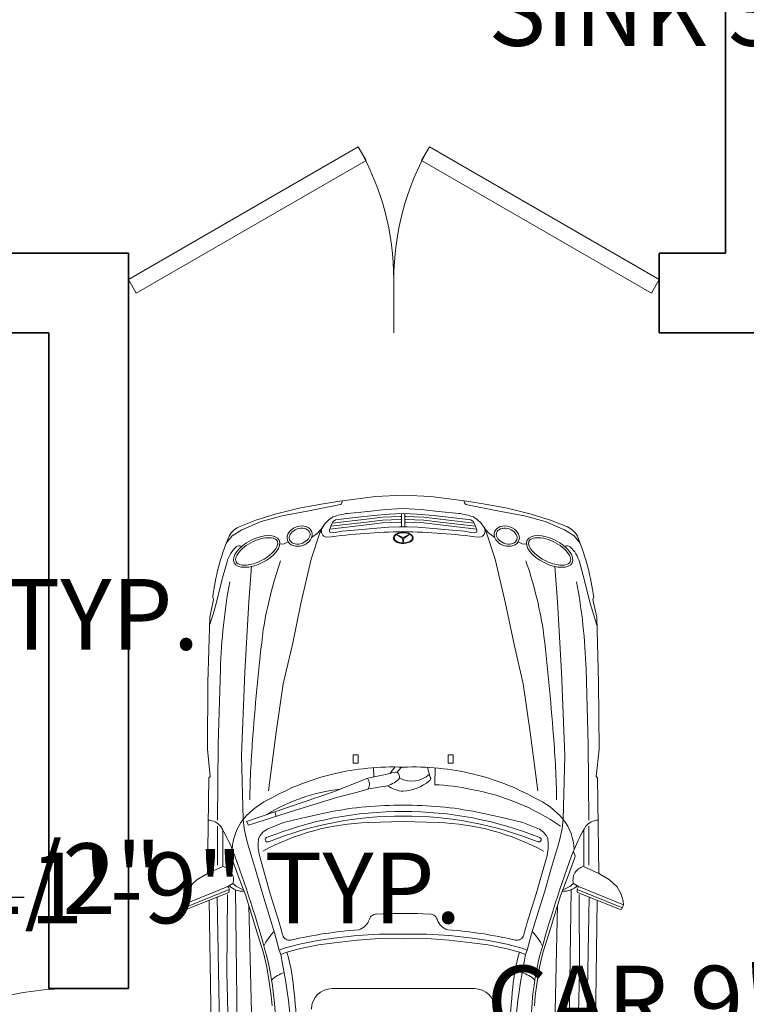
# Model space of a CAD drawing. Units: inches. Extents: x 2558 to 3026, y 433 to 1053.
# Tile 4 of 8: x 2795 to 2877, y 574 to 685. Entities that reach past the tile are written whole.
import ezdxf

# ---------------------------------------------------------------- set-up
doc = ezdxf.new("R2010")
doc.units = ezdxf.units.IN
for name, color, linetype, lineweight in [('0_Equip', 250, 'Continuous', 13), ('A-ANNO-DIMS', 2, 'Continuous', 18), ('A-DOOR', 4, 'Continuous', 18), ('A-WALL', 7, 'Continuous', 35)]:
    doc.layers.add(name, color=color, linetype=linetype, lineweight=lineweight)
doc.styles.get("Standard").update_dxf_attribs({"font": 'arial.ttf'})
doc.dimstyles.new('ISO-25', dxfattribs={"dimtxt": 8, "dimasz": 4, "dimexe": 1, "dimexo": 1, "dimgap": 1, "dimtad": 0, "dimtih": 1, "dimtoh": 1, "dimlunit": 3, "dimtxsty": 'Standard', "dimblk": 'OBLIQUE', "dimcen": 2.5, "dimclrt": 1, "dimadec": 0, "dimazin": 0, "dimtfac": 1, "dimtmove": 0, "dimatfit": 3, "dimfxl": 1, "dimfxlon": 1, "dimarcsym": 0})

# ---------------------------------------------------------------- blocks, each defined once
blk = doc.blocks.new('*U10')
for p, q in [((0, 0), (0, -6)), ((30, 0), (30, -6))]:
    blk.add_line(p, q)
blk.add_lwpolyline([(0, 0), (25.98, 15), (26.86, 13.48), (0.87, -1.52)], close=True)
blk.add_arc((0, 0), 30, 0, 30)
blk = doc.blocks.new('*U4')
for p, q in [((-30, 0), (-30, -6)), ((0, 0), (0, -6))]:
    blk.add_line(p, q)
blk.add_lwpolyline([(0, 0), (-25.98, 15), (-26.86, 13.48), (-0.88, -1.52)], close=True)
blk.add_arc((0, 0), 30, 150, 180)
blk = doc.blocks.new('*U8')
for p, q in [((0, 0), (0, -6)), ((36, 0), (36, -6))]:
    blk.add_line(p, q)
blk.add_lwpolyline([(0, 0), (31.18, 18), (32.05, 16.48), (0.87, -1.52)], close=True)
blk.add_arc((0, 0), 36, 0, 30)
blk = doc.blocks.new('A$C4C7B54D1')
at = {"layer": '0_Equip', "ltscale": 0.1}
for p, q in [((-0.7257, 2.678), (-0.8531, 2.6707)), ((-0.7257, 2.678), (-0.5983, 2.6707)), ((-1.112, 2.6343), (-1.2037, 2.6168)), ((-1.0138, 2.6343), (-1.1673, 2.6045)), ((-1.0176, 2.6505), (-1.112, 2.6343)), ((-0.8531, 2.6707), (-1.0176, 2.6505)), ((-0.5983, 2.6707), (-0.4338, 2.6505)), ((-0.4376, 2.6343), (-0.284, 2.6045)), ((-0.4338, 2.6505), (-0.3394, 2.6343)), ((-0.3394, 2.6343), (-0.2477, 2.6168)), ((-1.3142, 2.5898), (-1.4032, 2.5628)), ((-1.2824, 2.5829), (-1.3789, 2.557)), ((-1.2037, 2.6168), (-1.3142, 2.5898)), ((-1.1673, 2.6045), (-1.2824, 2.5829)), ((-0.8877, 2.6027), (-0.9812, 2.5937)), ((-0.8072, 2.6112), (-0.8877, 2.6027)), ((-0.7257, 2.6157), (-0.8072, 2.6112)), ((-0.7257, 2.6157), (-0.6441, 2.6112)), ((-0.6441, 2.6112), (-0.5636, 2.6027)), ((-0.5636, 2.6027), (-0.4701, 2.5937)), ((-0.284, 2.6045), (-0.1689, 2.5829)), ((-0.2477, 2.6168), (-0.1371, 2.5898)), ((-0.1689, 2.5829), (-0.0725, 2.557)), ((-0.1371, 2.5898), (-0.0481, 2.5628)), ((-1.4032, 2.5628), (-1.4801, 2.5318)), ((-1.3789, 2.557), (-1.4667, 2.5181)), ((-0.0725, 2.557), (0.0153, 2.5181)), ((-0.0481, 2.5628), (0.0288, 2.5318)), ((-1.5113, 2.4907), (-1.5393, 2.4562)), ((-1.4667, 2.5181), (-1.5113, 2.4907)), ((-1.1083, 2.5037), (-1.1486, 2.3827)), ((-0.343, 2.5037), (-0.3027, 2.3827)), ((0.0153, 2.5181), (0.06, 2.4907)), ((0.06, 2.4907), (0.0879, 2.4562)), ((-1.5353, 2.3701), (-1.5529, 2.308)), ((-1.1486, 2.3827), (-1.1961, 2.1797)), ((-0.3027, 2.3827), (-0.2552, 2.1797)), ((0.084, 2.3701), (0.1016, 2.308)), ((-1.435, 2.1869), (-1.4221, 2.3511)), ((-0.0163, 2.1869), (-0.0293, 2.3511)), ((-1.5529, 2.308), (-1.5677, 2.2486)), ((0.1016, 2.308), (0.1164, 2.2486)), ((-1.5677, 2.2486), (-1.5849, 2.1795)), ((0.1164, 2.2486), (0.1336, 2.1795)), ((-1.597, 2.1976), (-1.615, 2.1169)), ((-1.6012, 2.2082), (-1.597, 2.1976)), ((-1.5849, 2.1795), (-1.5997, 2.1304)), ((-1.4537, 1.863), (-1.435, 2.1869)), ((-1.1961, 2.1797), (-1.2349, 1.9911)), ((-0.2552, 2.1797), (-0.2164, 1.9911)), ((0.0024, 1.863), (-0.0163, 2.1869)), ((0.1336, 2.1795), (0.1484, 2.1304)), ((0.1499, 2.2082), (0.1457, 2.1976)), ((0.1457, 2.1976), (0.1637, 2.1169)), ((-1.5997, 2.1304), (-1.6161, 2.0798)), ((0.1484, 2.1304), (0.1647, 2.0798)), ((-1.615, 2.1169), (-1.6235, 1.8165)), ((0.1637, 2.1169), (0.1722, 1.8165)), ((-1.2349, 1.9911), (-1.2767, 1.8097)), ((-0.2164, 1.9911), (-0.1746, 1.8097)), ((-1.566, 1.8774), (-1.5761, 1.5304)), ((-1.4681, 1.48), (-1.4537, 1.863)), ((0.0168, 1.48), (0.0024, 1.863)), ((0.1147, 1.8774), (0.1247, 1.5304)), ((-1.6235, 1.8165), (-1.6256, 1.5098)), ((0.1722, 1.8165), (0.1743, 1.5098)), ((-1.2767, 1.8097), (-1.3098, 1.588)), ((-0.1746, 1.8097), (-0.1415, 1.588)), ((-1.3098, 1.588), (-1.3443, 1.3187)), ((-0.1415, 1.588), (-0.107, 1.3187)), ((-1.6256, 1.5098), (-1.6129, 1.3846)), ((-1.5761, 1.5304), (-1.5789, 1.1834)), ((0.1247, 1.5304), (0.1276, 1.1834)), ((0.1743, 1.5098), (0.1616, 1.3846)), ((-1.461, 1.1868), (-1.4681, 1.48)), ((-0.955, 1.4459), (-0.955, 1.4827)), ((-0.955, 1.4827), (-0.9321, 1.4827)), ((-0.9321, 1.4827), (-0.9321, 1.4459)), ((-0.5192, 1.4827), (-0.5192, 1.4459)), ((-0.4964, 1.4827), (-0.5192, 1.4827)), ((-0.4964, 1.4459), (-0.4964, 1.4827)), ((0.0097, 1.1868), (0.0168, 1.48)), ((-0.9321, 1.4459), (-0.955, 1.4459)), ((-0.8614, 1.4242), (-0.8603, 1.382)), ((-0.6135, 1.4258), (-0.6012, 1.3814)), ((-0.5809, 1.3459), (-0.5793, 1.4233)), ((-0.5192, 1.4459), (-0.4964, 1.4459)), ((-1.6193, 1.3782), (-1.6252, 0.9375)), ((-1.6129, 1.3846), (-1.6193, 1.3782)), ((-0.8878, 1.3764), (-1.0456, 1.313)), ((-0.7861, 1.3973), (-0.8878, 1.3764)), ((0.1616, 1.3846), (0.1679, 1.3782)), ((0.1679, 1.3782), (0.1739, 0.9375)), ((-1.0456, 1.313), (-1.4462, 1.1776)), ((-0.9361, 1.3119), (-0.8835, 1.3269)), ((-0.8835, 1.3269), (-0.7975, 1.3408)), ((-1.2207, 1.2292), (-1.0263, 1.2883)), ((-1.0263, 1.2883), (-0.9361, 1.3119)), ((-1.4366, 1.1604), (-1.2207, 1.2292)), ((-1.4565, 1.1447), (-1.461, 1.1868)), ((-1.4462, 1.1776), (-1.4366, 1.1604)), ((-1.3162, 1.2215), (-1.3088, 1.2011)), ((-1.1723, 1.1976), (-1.2762, 1.1716)), ((-1.0667, 1.22), (-1.1723, 1.1976)), ((-0.7257, 1.1776), (-0.8858, 1.1725)), ((-0.7257, 1.1776), (-0.5655, 1.1725)), ((-0.3847, 1.22), (-0.279, 1.1976)), ((-0.279, 1.1976), (-0.1751, 1.1716)), ((0.0052, 1.1447), (0.0097, 1.1868)), ((-1.5793, 1.1562), (-1.5793, 0.9761)), ((-1.5552, 1.139), (-1.5552, 0.9693)), ((-1.4503, 1.1151), (-1.4565, 1.1447)), ((-1.3515, 1.142), (-1.3703, 1.1286)), ((-1.2762, 1.1716), (-1.3515, 1.142)), ((-0.1751, 1.1716), (-0.0999, 1.142)), ((-0.0999, 1.142), (-0.0811, 1.1286)), ((-0.0011, 1.1151), (0.0052, 1.1447)), ((0.1038, 1.139), (0.1038, 0.9693)), ((0.128, 1.1562), (0.128, 0.9761)), ((-1.444, 1.0892), (-1.4503, 1.1151)), ((-1.4368, 1.0623), (-1.444, 1.0892)), ((-1.39, 1.0981), (-1.3927, 1.0739)), ((-1.3828, 1.1133), (-1.39, 1.0981)), ((-1.3703, 1.1286), (-1.3828, 1.1133)), ((-0.0811, 1.1286), (-0.0685, 1.1133)), ((-0.0685, 1.1133), (-0.0614, 1.0981)), ((-0.0614, 1.0981), (-0.0587, 1.0739)), ((-0.0145, 1.0623), (-0.0073, 1.0892)), ((-0.0073, 1.0892), (-0.0011, 1.1151)), ((-1.4243, 1.0229), (-1.4368, 1.0623)), ((-1.3927, 1.0739), (-1.3918, 1.0533)), ((-1.3918, 1.0533), (-1.3867, 1.0211)), ((-0.0596, 1.0533), (-0.0646, 1.0211)), ((-0.0587, 1.0739), (-0.0596, 1.0533)), ((-0.027, 1.0229), (-0.0145, 1.0623)), ((-1.5149, 1.011), (-1.4844, 0.9277)), ((-1.4064, 0.961), (-1.4243, 1.0229)), ((-1.3867, 1.0211), (-1.3374, 0.8446)), ((-0.0646, 1.0211), (-0.1139, 0.8446)), ((-0.0449, 0.961), (-0.027, 1.0229)), ((0.0635, 1.011), (0.0331, 0.9277)), ((-1.6252, 0.9375), (-1.5546, 0.9696)), ((-1.3759, 0.8562), (-1.4064, 0.961)), ((-0.0754, 0.8562), (-0.0449, 0.961)), ((0.1739, 0.9375), (0.1032, 0.9696)), ((-1.6745, 0.908), (-1.7088, 0.8764)), ((-1.6252, 0.9375), (-1.6745, 0.908)), ((-1.4844, 0.9277), (-1.4486, 0.8345)), ((0.0331, 0.9277), (-0.0028, 0.8345)), ((0.1739, 0.9375), (0.2232, 0.908)), ((0.2232, 0.908), (0.2574, 0.8764)), ((-1.5321, 0.8786), (-1.7381, 0.7945)), ((-1.5253, 0.865), (-1.7329, 0.7802)), ((-1.7088, 0.8764), (-1.728, 0.8432)), ((-1.508, 0.8914), (-1.5321, 0.8786)), ((-1.4835, -0.0735), (-1.497, 0.863)), ((0.0322, -0.0735), (0.0457, 0.863)), ((0.0566, 0.8914), (0.0807, 0.8786)), ((0.074, 0.865), (0.2816, 0.7802)), ((0.0807, 0.8786), (0.2867, 0.7945)), ((0.2574, 0.8764), (0.2767, 0.8432)), ((-1.728, 0.8432), (-1.7366, 0.8127)), ((-1.5273, 0.8512), (-1.7203, 0.7738)), ((-1.6171, 0.8152), (-1.5964, -0.6171)), ((-1.5805, 0.8299), (-1.5623, -0.138)), ((-1.5337, 0.8406), (-1.5355, 0.484)), ((-1.4486, 0.8345), (-1.4226, 0.7503)), ((-1.3401, 0.7406), (-1.3759, 0.8562)), ((-1.3374, 0.8446), (-1.3097, 0.7577)), ((-0.1139, 0.8446), (-0.1417, 0.7577)), ((-0.1112, 0.7406), (-0.0754, 0.8562)), ((-0.0028, 0.8345), (-0.0287, 0.7503)), ((0.0759, 0.8512), (0.269, 0.7738)), ((0.0824, 0.8406), (0.0842, 0.484)), ((0.1292, 0.8299), (0.111, -0.138)), ((0.1658, 0.8152), (0.145, -0.6171)), ((0.2767, 0.8432), (0.2853, 0.8127)), ((-1.7366, 0.8127), (-1.7377, 0.7934)), ((-1.7377, 0.7934), (-1.7327, 0.7794)), ((-1.4352, 0.792), (-1.4152, -0.045)), ((-0.0162, 0.792), (-0.0361, -0.045)), ((0.2863, 0.7934), (0.2813, 0.7794)), ((0.2853, 0.8127), (0.2863, 0.7934)), ((-1.4226, 0.7503), (-1.4029, 0.6849)), ((-1.315, 0.66), (-1.3401, 0.7406)), ((-1.3097, 0.7577), (-1.2953, 0.7129)), ((-0.7926, 0.7532), (-0.8418, 0.7514)), ((-0.7257, 0.7541), (-0.7926, 0.7532)), ((-0.7257, 0.7541), (-0.6587, 0.7532)), ((-0.6587, 0.7532), (-0.6095, 0.7514)), ((-0.1417, 0.7577), (-0.156, 0.7129)), ((-0.1363, 0.66), (-0.1112, 0.7406)), ((-0.0287, 0.7503), (-0.0484, 0.6849)), ((-1.4029, 0.6849), (-1.368, 0.5729)), ((-1.2953, 0.7129), (-1.2801, 0.6573)), ((-0.156, 0.7129), (-0.1712, 0.6573)), ((-0.0484, 0.6849), (-0.0834, 0.5729)), ((-1.2951, 0.5849), (-1.315, 0.66)), ((-1.2801, 0.6573), (-1.2795, 0.6546)), ((-1.0437, 0.6403), (-1.1177, 0.6302)), ((-0.9389, 0.6526), (-1.0437, 0.6403)), ((-0.8346, 0.6593), (-0.9389, 0.6526)), ((-0.834, 0.6384), (-0.937, 0.6317)), ((-0.7257, 0.6582), (-0.8346, 0.6593)), ((-0.7257, 0.6373), (-0.834, 0.6384)), ((-0.7257, 0.6582), (-0.6168, 0.6593)), ((-0.7257, 0.6373), (-0.6173, 0.6384)), ((-0.6173, 0.6384), (-0.5143, 0.6317)), ((-0.6168, 0.6593), (-0.5124, 0.6526)), ((-0.5124, 0.6526), (-0.4076, 0.6403)), ((-0.4076, 0.6403), (-0.3337, 0.6302)), ((-0.1712, 0.6573), (-0.1719, 0.6546)), ((-0.1562, 0.5849), (-0.1363, 0.66)), ((-1.2663, 0.5956), (-1.2951, 0.5849)), ((-1.2021, 0.6133), (-1.2663, 0.5956)), ((-1.1973, 0.593), (-1.2599, 0.5757)), ((-1.1177, 0.6302), (-1.2021, 0.6133)), ((-1.1142, 0.6096), (-1.1973, 0.593)), ((-1.0411, 0.6196), (-1.1142, 0.6096)), ((-0.937, 0.6317), (-1.0411, 0.6196)), ((-0.5143, 0.6317), (-0.4102, 0.6196)), ((-0.4102, 0.6196), (-0.3371, 0.6096)), ((-0.3371, 0.6096), (-0.2541, 0.593)), ((-0.3337, 0.6302), (-0.2492, 0.6133)), ((-0.2541, 0.593), (-0.1914, 0.5757)), ((-0.2492, 0.6133), (-0.185, 0.5956)), ((-0.185, 0.5956), (-0.1562, 0.5849)), ((-1.368, 0.5729), (-1.3527, 0.5066)), ((-1.2879, 0.5653), (-1.2951, 0.5849)), ((-1.2599, 0.5757), (-1.2879, 0.5653)), ((-0.1914, 0.5757), (-0.1635, 0.5653)), ((-0.1635, 0.5653), (-0.1562, 0.5849)), ((-0.0834, 0.5729), (-0.0986, 0.5066)), ((-1.3527, 0.5066), (-1.3411, 0.4394)), ((-0.0986, 0.5066), (-0.1102, 0.4394)), ((-1.5355, 0.484), (-1.5292, 0.2045)), ((0.0842, 0.484), (0.0779, 0.2045)), ((-1.3411, 0.4394), (-1.3321, 0.3749)), ((-0.7257, 0.4085), (-1.0528, 0.4085)), ((-0.7257, 0.4085), (-0.3986, 0.4085)), ((-0.1102, 0.4394), (-0.1192, 0.3749)), ((-1.3321, 0.3749), (-1.3286, 0.3301)), ((-0.1192, 0.3749), (-0.1228, 0.3301)), ((-1.3178, 0.3418), (-1.31, 0.2426)), ((-0.1335, 0.3418), (-0.1413, 0.2426))]:
    blk.add_line(p, q, dxfattribs=at)
at = {"layer": '0_Equip'}
for p, q in [((-0.8628, 2.5838), (-0.9467, 2.5739)), ((-0.7905, 2.5897), (-0.8628, 2.5838)), ((-0.7257, 2.5926), (-0.7905, 2.5897)), ((-0.733, 2.5923), (-0.733, 2.5325)), ((-0.7257, 2.5926), (-0.6608, 2.5897)), ((-0.7183, 2.5923), (-0.7183, 2.5325)), ((-0.6608, 2.5897), (-0.5886, 2.5838)), ((-0.5886, 2.5838), (-0.5046, 2.5739)), ((-1.0545, 2.5425), (-1.0638, 2.5185)), ((-1.0631, 2.5204), (-0.8949, 2.5405)), ((-1.0577, 2.5343), (-0.8949, 2.5537)), ((-1.0475, 2.557), (-1.0545, 2.5425)), ((-1.0517, 2.5482), (-0.8949, 2.567)), ((-1.0364, 2.5634), (-1.0475, 2.557)), ((-0.9467, 2.5739), (-1.0364, 2.5634)), ((-0.8949, 2.567), (-0.8211, 2.5763)), ((-0.8949, 2.5537), (-0.8211, 2.5631)), ((-0.8949, 2.5405), (-0.8211, 2.5498)), ((-0.8211, 2.5763), (-0.738, 2.5791)), ((-0.8211, 2.5631), (-0.738, 2.5659)), ((-0.8211, 2.5498), (-0.738, 2.5526)), ((-0.738, 2.5791), (-0.733, 2.58)), ((-0.738, 2.5659), (-0.733, 2.5668)), ((-0.738, 2.5526), (-0.733, 2.5536)), ((-0.7133, 2.5791), (-0.7183, 2.58)), ((-0.7133, 2.5659), (-0.7183, 2.5668)), ((-0.7133, 2.5526), (-0.7183, 2.5536)), ((-0.6302, 2.5763), (-0.7133, 2.5791)), ((-0.6302, 2.5631), (-0.7133, 2.5659)), ((-0.6302, 2.5498), (-0.7133, 2.5526)), ((-0.5564, 2.567), (-0.6302, 2.5763)), ((-0.5564, 2.5537), (-0.6302, 2.5631)), ((-0.5564, 2.5405), (-0.6302, 2.5498)), ((-0.3996, 2.5482), (-0.5564, 2.567)), ((-0.3936, 2.5343), (-0.5564, 2.5537)), ((-0.3882, 2.5204), (-0.5564, 2.5405)), ((-0.5046, 2.5739), (-0.4149, 2.5634)), ((-0.4149, 2.5634), (-0.4038, 2.557)), ((-0.4038, 2.557), (-0.3968, 2.5425)), ((-0.3968, 2.5425), (-0.3875, 2.5185)), ((-1.0638, 2.5185), (-1.0638, 2.5092)), ((-1.0638, 2.5092), (-1.0545, 2.504)), ((-1.0545, 2.504), (-1.0376, 2.5051)), ((-1.0376, 2.5051), (-1.0067, 2.5116)), ((-1.0067, 2.5116), (-0.9502, 2.5168)), ((-0.9502, 2.5168), (-0.8657, 2.5238)), ((-0.8657, 2.5238), (-0.7922, 2.5308)), ((-0.7922, 2.5308), (-0.7433, 2.5325)), ((-0.7566, 2.4971), (-0.7261, 2.4828)), ((-0.7566, 2.4971), (-0.7291, 2.4776)), ((-0.7433, 2.5325), (-0.7257, 2.5325)), ((-0.7389, 2.5095), (-0.7395, 2.5059)), ((-0.6947, 2.4974), (-0.7261, 2.4828)), ((-0.708, 2.5325), (-0.7257, 2.5325)), ((-0.6947, 2.4974), (-0.723, 2.4776)), ((-0.7124, 2.5095), (-0.7119, 2.5059)), ((-0.6591, 2.5308), (-0.708, 2.5325)), ((-0.5857, 2.5238), (-0.6591, 2.5308)), ((-0.5011, 2.5168), (-0.5857, 2.5238)), ((-0.4446, 2.5116), (-0.5011, 2.5168)), ((-0.4137, 2.5051), (-0.4446, 2.5116)), ((-0.3968, 2.504), (-0.4137, 2.5051)), ((-0.3875, 2.5092), (-0.3968, 2.504)), ((-0.3875, 2.5185), (-0.3875, 2.5092)), ((-0.7259, 2.4578), (-0.7291, 2.4776)), ((-0.7259, 2.4578), (-0.723, 2.4776))]:
    blk.add_line(p, q, dxfattribs=at)
at = {"layer": '0_Equip', "ltscale": 0.1}
for centre, radius, start, end in [((-1.0252, 2.6508), 0.02, 304.7228, 3.5172), ((-0.4261, 2.6508), 0.02, 176.4828, 235.2772), ((-0.9299, 2.2354), 0.3619, 98.1466, 109.2524), ((-0.5214, 2.2354), 0.3619, 70.7476, 81.8534), ((-0.9799, 2.461), 0.1353, 120.8369, 151.2853), ((-0.4714, 2.461), 0.1353, 28.7147, 59.1631), ((-1.4391, 2.4422), 0.0986, 114.5945, 157.5113), ((-1.2153, 2.6098), 0.1432, 299.1564, 328.1831), ((-0.9799, 2.461), 0.1353, 151.2853, 161.5889), ((-1.0728, 2.5126), 0.029, 152.6038, 261.721), ((-0.6679, -0.6671), 3.1773, 91.0415, 97.3969), ((-0.7834, -0.6671), 3.1773, 82.6031, 88.9585), ((-0.3785, 2.5126), 0.029, 278.279, 27.3962), ((-0.236, 2.6098), 0.1432, 211.8169, 240.8436), ((-0.4714, 2.461), 0.1353, 18.4111, 28.7147), ((-0.0123, 2.4422), 0.0986, 22.4887, 65.4055), ((-0.4722, 2.0579), 1.139, 158.2564, 172.4203), ((-1.2841, 2.5028), 0.0501, 260.5448, 306.7068), ((-0.1672, 2.5028), 0.0501, 233.2932, 279.4552), ((-0.9791, 2.0579), 1.139, 7.5797, 21.7436), ((-1.4083, 2.3394), 0.1306, 130.2084, 166.4224), ((-1.4798, 2.4259), 0.0184, 54.8052, 134.0204), ((0.0285, 2.4259), 0.0184, 45.9796, 125.1948), ((-0.043, 2.3394), 0.1306, 13.5776, 49.7916), ((0.5502, 1.746), 1.9445, 161.1117, 170.7019), ((-2.0015, 1.746), 1.9445, 9.2981, 18.8883), ((1.1202, 1.7918), 2.6875, 169.5541, 178.1755), ((-2.5715, 1.7918), 2.6875, 1.8245, 10.4459), ((9.2655, 0.7813), 10.7109, 173.14258, 175.77374), ((-10.7169, 0.7813), 10.7109, 4.22626, 6.85742), ((2.9623, 1.2089), 4.3935, 175.2767, 179.1124), ((-4.4136, 1.2089), 4.3935, 0.8876, 4.7233), ((-0.7686, 0.201), 1.2267, 87.9955, 103.2364), ((-0.3726, 1.0935), 0.5131, 139.3585, 143.6922), ((-0.7554, 1.327), 0.0768, 88.1186, 113.6019), ((-0.6528, 1.3354), 0.1211, 130.7679, 145.6911), ((-0.7803, 1.3768), 0.0384, 357.9275, 44.3829), ((-0.6828, 0.201), 1.2267, 76.7636, 92.0045), ((-0.786, 0.3109), 1.1158, 103.6551, 119.1148), ((-0.9216, 1.3498), 0.0409, 323.4512, 39.0343), ((-0.8494, 1.486), 0.1542, 289.6676, 314.192), ((-0.6872, 1.4869), 0.1241, 243.8649, 311.6638), ((-0.741, 1.5272), 0.212, 274.1513, 309.4931), ((-0.6113, 1.3746), 0.0122, 294.8678, 33.6398), ((-0.6653, 0.3109), 1.1158, 60.8852, 76.3449), ((-0.929, 0.5266), 0.803, 96.22, 121.6991), ((-0.7147, 1.4628), 0.1474, 235.8143, 265.7174), ((-0.617, 0.3882), 0.9584, 77.6919, 87.8428), ((-0.5976, 0.2949), 1.0461, 55.3038, 79.8165), ((-1.1803, 0.9494), 0.3676, 113.8511, 139.7847), ((-0.2711, 0.9494), 0.3676, 40.2153, 66.1489), ((-0.7356, -0.4312), 1.6538, 89.6554, 111.9286), ((-0.7478, -0.378), 1.6295, 89.2231, 101.2856), ((-0.7036, -0.378), 1.6295, 78.7144, 90.7769), ((-0.7157, -0.4312), 1.6538, 68.0714, 90.3446), ((-1.6261, 1.102), 0.0813, 40.278, 87.0689), ((-1.2706, 1.0395), 0.2408, 142.2718, 177.7746), ((-0.7356, -0.4312), 1.6329, 89.6554, 111.9286), ((-0.7157, -0.4312), 1.6329, 68.0714, 90.3446), ((-0.1807, 1.0395), 0.2408, 2.2254, 37.7282), ((0.1747, 1.102), 0.0813, 92.9311, 139.722), ((-2.3477, 0.6968), 0.9076, 22.824, 30.2904), ((-0.85, 0.0855), 1.0875, 91.8892, 118.6013), ((-0.6014, 0.0855), 1.0875, 61.3987, 88.1108), ((0.8964, 0.6968), 0.9076, 149.7096, 157.176), ((-1.3493, 1.0932), 0.0105, 111.9286, 291.9286), ((-0.102, 1.0932), 0.0105, 248.0714, 68.0714), ((-6.6059, -0.8606), 5.4408, 15.0904, 20.5451), ((5.1546, -0.8606), 5.4408, 159.4549, 164.9096), ((-1.4887, 1.0171), 0.0269, 132.3277, 193.1064), ((0.0373, 1.0171), 0.0269, 346.8936, 47.6723), ((-1.5684, 0.9084), 0.0628, 344.3283, 77.2348), ((0.1171, 0.9084), 0.0628, 102.7652, 195.6717), ((-1.5495, 0.8614), 0.0245, 335.4987, 44.5114), ((-1.463, 0.9441), 0.0879, 224.7932, 273.9292), ((-1.4233, 0.9849), 0.1262, 227.8287, 253.081), ((0.0117, 0.9441), 0.0879, 266.0708, 315.2068), ((-0.0281, 0.9849), 0.1262, 286.919, 312.1713), ((0.0982, 0.8614), 0.0245, 135.4886, 204.5013), ((-1.7238, 0.7825), 0.00941, 199.646, 291.8616), ((0.2725, 0.7825), 0.00941, 248.1384, 340.354), ((-0.9515, 0.7495), 0.0737, 286.567, 342.4011), ((-0.8474, 0.7163), 0.0355, 80.937, 162.15), ((-0.6039, 0.7163), 0.0355, 17.85, 99.063), ((-0.4998, 0.7495), 0.0737, 197.5989, 253.433), ((-1.1535, 0.5061), 0.2334, 134.9877, 155.4049), ((-1.249, 0.662), 0.0314, 193.667, 283.2045), ((-0.7896, -1.2957), 1.9795, 94.0807, 103.2045), ((-0.6617, -1.2957), 1.9795, 76.7955, 85.9193), ((-0.2023, 0.662), 0.0314, 256.7955, 346.333), ((-0.2978, 0.5061), 0.2334, 24.5951, 45.0123), ((-2.6334, 0.2371), 1.3197, 4.5498, 13.9797), ((-4.2099, -0.0242), 2.9809, 358.1905, 11.4064), ((-2.0025, 0.3511), 0.7759, 4.7259, 16.8296), ((2.7585, -0.0242), 2.9809, 168.5936, 181.8095), ((0.5512, 0.3511), 0.7759, 163.1704, 175.2741), ((1.1821, 0.2371), 1.3197, 166.0203, 175.4502), ((-1.2324, 0.3484), 0.1397, 106.6168, 134.6647), ((-0.2189, 0.3484), 0.1397, 45.3353, 73.3832), ((-6.5594, -0.126), 5.3575, 1.3159, 5.7952), ((-1.0528, 0.3145), 0.0941, 90, 180), ((-0.3986, 0.3145), 0.0941, 0, 90), ((5.1081, -0.126), 5.3575, 174.2048, 178.6841)]:
    blk.add_arc(centre, radius, start, end, dxfattribs=at)
for centre, major_axis, ratio in [((-1.2016, 2.4892), (0.0562, 0.0189), 0.759763), ((-1.399, 2.4187), (-0.1036, -0.0518), 0.497493)]:
    blk.add_ellipse(centre, major_axis=major_axis, ratio=ratio, dxfattribs=at)
at = {"layer": '0_Equip', "ltscale": 0.1, "extrusion": (0, 0, -1)}
for centre, major_axis, ratio in [((-0.2497, 2.4892), (-0.0562, 0.0189), 0.759763), ((-0.0523, 2.4187), (0.1036, -0.0518), 0.497493)]:
    blk.add_ellipse(centre, major_axis=major_axis, ratio=ratio, dxfattribs=at)
at = {"layer": '0_Equip'}
blk.add_ellipse((-0.7253, 2.4812), major_axis=(-0.0426, 0), ratio=0.550187, dxfattribs=at)
at = {"layer": '0_Equip', "ltscale": 0.1}
for points, knots in [([(-1.1548, 2.5048), (-1.1596, 2.5191), (-1.1811, 2.5294), (-1.2283, 2.5198), (-1.248, 2.5001), (-1.2511, 2.4679), (-1.2373, 2.4539), (-1.1922, 2.4512), (-1.1656, 2.4658), (-1.1532, 2.4906), (-1.1526, 2.4983), (-1.1548, 2.5048)], [0, 0, 0, 0, 1.408119, 1.408119, 2.816238, 2.816238, 4.224358, 4.224358, 5.632477, 5.632477, 6.283185, 6.283185, 6.283185, 6.283185]), ([(-0.2965, 2.5048), (-0.2917, 2.5191), (-0.2703, 2.5294), (-0.2231, 2.5198), (-0.2033, 2.5001), (-0.2003, 2.4679), (-0.2141, 2.4539), (-0.2592, 2.4512), (-0.2858, 2.4658), (-0.2981, 2.4906), (-0.2987, 2.4983), (-0.2965, 2.5048)], [0, 0, 0, 0, 1.408119, 1.408119, 2.816238, 2.816238, 4.224358, 4.224358, 5.632477, 5.632477, 6.283185, 6.283185, 6.283185, 6.283185]), ([(-1.4937, 2.3714), (-1.4901, 2.3641), (-1.4809, 2.3581), (-1.4492, 2.3543), (-1.4277, 2.3571), (-1.3679, 2.3771), (-1.3298, 2.404), (-1.2994, 2.4483), (-1.2993, 2.4626), (-1.3171, 2.4801), (-1.3406, 2.4849), (-1.3989, 2.4733), (-1.4323, 2.4577), (-1.4816, 2.4186), (-1.4956, 2.3954), (-1.4959, 2.3774), (-1.4951, 2.3742), (-1.4937, 2.3714)], [0, 0, 0, 0, 0.646556, 0.646556, 1.293113, 1.293113, 2.410172, 2.410172, 3.309931, 3.309931, 4.20969, 4.20969, 5.109449, 5.109449, 6.031285, 6.031285, 6.283185, 6.283185, 6.283185, 6.283185]), ([(0.0424, 2.3714), (0.0388, 2.3641), (0.0295, 2.3581), (-0.0022, 2.3543), (-0.0236, 2.3571), (-0.0834, 2.3771), (-0.1216, 2.404), (-0.152, 2.4483), (-0.152, 2.4626), (-0.1343, 2.4801), (-0.1108, 2.4849), (-0.0524, 2.4733), (-0.019, 2.4577), (0.0303, 2.4186), (0.0443, 2.3954), (0.0445, 2.3774), (0.0438, 2.3742), (0.0424, 2.3714)], [0, 0, 0, 0, 0.646556, 0.646556, 1.293113, 1.293113, 2.410172, 2.410172, 3.309931, 3.309931, 4.20969, 4.20969, 5.109449, 5.109449, 6.031285, 6.031285, 6.283185, 6.283185, 6.283185, 6.283185])]:
    blk.add_open_spline(points, degree=3, knots=knots, dxfattribs=at)
at = {"layer": '0_Equip'}
blk.add_open_spline([(-0.7708, 2.4812), (-0.7708, 2.4725), (-0.7635, 2.4648), (-0.7294, 2.4499), (-0.6897, 2.4563), (-0.6733, 2.4916), (-0.7036, 2.5102), (-0.7526, 2.5051), (-0.7708, 2.4948), (-0.7708, 2.4812)], degree=3, knots=[0, 0, 0, 0, 0.903923, 0.903923, 2.878844, 2.878844, 4.872977, 4.872977, 6.283185, 6.283185, 6.283185, 6.283185], dxfattribs=at)
blk = doc.blocks.new('_Oblique')
at = {"color": 0, "linetype": 'ByBlock', "lineweight": -2}
blk.add_line((-0.5, -0.5), (0.5, 0.5), dxfattribs=at)
blk = doc.blocks.new('*D27')
at = {"layer": 'A-ANNO-DIMS', "color": 0, "lineweight": -2, "transparency": 16777216}
for p, q in [((2764.96, 640.74), (2762.96, 640.74)), ((2763.96, 640.74), (2763.96, 622.08)), ((2763.96, 593.15), (2763.96, 611.8)), ((2764.96, 593.15), (2762.96, 593.15))]:
    blk.add_line(p, q, dxfattribs=at)
at = {"layer": 'Defpoints', "color": 0, "transparency": 16777216}
for p in [(2771.1, 640.74), (2763.96, 593.15), (2771.1, 593.15)]:
    blk.add_point(p, dxfattribs=at)
at = {"layer": 'A-ANNO-DIMS', "color": 0, "lineweight": -2, "transparency": 16777216, "xscale": 4, "yscale": 4, "zscale": 4}
for p, rotation in [((2763.96, 640.74), 90), ((2763.96, 593.15), 270)]:
    blk.add_blockref('_Oblique', p, dxfattribs=dict(at, rotation=rotation))
at = {"layer": 'A-ANNO-DIMS', "color": 1, "transparency": 16777216, "insert": (2763.96, 616.94), "char_height": 8, "attachment_point": 5}
blk.add_mtext('SOFA 3\'-11 1/2" TYP.', dxfattribs=at)
blk = doc.blocks.new('*D28')
at = {"layer": 'A-ANNO-DIMS', "color": 0, "lineweight": -2, "transparency": 16777216}
for p, q in [((2771.1, 587.01), (2771.1, 585.01)), ((2791.87, 587.01), (2791.87, 585.01)), ((2771.1, 586.01), (2791.87, 586.01)), ((2791.87, 586.01), (2795.87, 586.01))]:
    blk.add_line(p, q, dxfattribs=at)
at = {"layer": 'Defpoints', "color": 0, "transparency": 16777216}
for p in [(2771.1, 593.15), (2791.87, 593.15), (2791.87, 586.01)]:
    blk.add_point(p, dxfattribs=at)
at = {"layer": 'A-ANNO-DIMS', "color": 0, "lineweight": -2, "transparency": 16777216, "xscale": 4, "yscale": 4, "zscale": 4, "rotation": 180}
blk.add_blockref('_Oblique', (2771.1, 586.01), dxfattribs=at)
at = {"layer": 'A-ANNO-DIMS', "color": 0, "lineweight": -2, "transparency": 16777216, "xscale": 4, "yscale": 4, "zscale": 4}
blk.add_blockref('_Oblique', (2791.87, 586.01), dxfattribs=at)
at = {"layer": 'A-ANNO-DIMS', "color": 1, "transparency": 16777216, "insert": (2820.88, 586.01), "char_height": 8, "attachment_point": 5}
blk.add_mtext('1\'-9" TYP.', dxfattribs=at)
blk = doc.blocks.new('*D34')
at = {"layer": 'A-ANNO-DIMS', "color": 0, "lineweight": -2, "transparency": 16777216}
for p, q in [((2743.78, 588.05), (2743.78, 586.05)), ((2765.34, 588.05), (2765.34, 586.05)), ((2743.78, 587.05), (2765.34, 587.05)), ((2765.34, 587.05), (2769.34, 587.05))]:
    blk.add_line(p, q, dxfattribs=at)
at = {"layer": 'Defpoints', "color": 0, "transparency": 16777216}
for p in [(2743.78, 593.52), (2765.34, 593.52), (2765.34, 587.05)]:
    blk.add_point(p, dxfattribs=at)
at = {"layer": 'A-ANNO-DIMS', "color": 0, "lineweight": -2, "transparency": 16777216, "xscale": 4, "yscale": 4, "zscale": 4, "rotation": 180}
blk.add_blockref('_Oblique', (2743.78, 587.05), dxfattribs=at)
at = {"layer": 'A-ANNO-DIMS', "color": 0, "lineweight": -2, "transparency": 16777216, "xscale": 4, "yscale": 4, "zscale": 4}
blk.add_blockref('_Oblique', (2765.34, 587.05), dxfattribs=at)
at = {"layer": 'A-ANNO-DIMS', "color": 1, "transparency": 16777216, "insert": (2789.92, 587.05), "char_height": 8, "attachment_point": 5}
blk.add_mtext('1\'-9 1/2"', dxfattribs=at)
blk = doc.blocks.new('*D41')
at = {"layer": 'A-ANNO-DIMS', "color": 0, "lineweight": -2, "transparency": 16777216}
for p, q in [((2904.13, 684.22), (2904.13, 686.22)), ((2940.13, 684.22), (2940.13, 686.22)), ((2904.13, 685.22), (2900.13, 685.22)), ((2940.13, 685.22), (2904.13, 685.22))]:
    blk.add_line(p, q, dxfattribs=at)
at = {"layer": 'Defpoints', "color": 0, "transparency": 16777216}
for p in [(2904.13, 685.22), (2904.13, 679.82), (2940.13, 679.82)]:
    blk.add_point(p, dxfattribs=at)
at = {"layer": 'A-ANNO-DIMS', "color": 0, "lineweight": -2, "transparency": 16777216, "xscale": 4, "yscale": 4, "zscale": 4, "rotation": 180}
blk.add_blockref('_Oblique', (2904.13, 685.22), dxfattribs=at)
at = {"layer": 'A-ANNO-DIMS', "color": 0, "lineweight": -2, "transparency": 16777216, "xscale": 4, "yscale": 4, "zscale": 4}
blk.add_blockref('_Oblique', (2940.13, 685.22), dxfattribs=at)
at = {"layer": 'A-ANNO-DIMS', "color": 1, "transparency": 16777216, "insert": (2873.92, 685.22), "char_height": 8, "attachment_point": 5}
blk.add_mtext('SINK 3\'-0"', dxfattribs=at)
blk = doc.blocks.new('*D43')
at = {"layer": 'A-ANNO-DIMS', "color": 0, "lineweight": -2, "transparency": 16777216}
for p, q in [((2880.07, 631.47), (2882.07, 631.47)), ((2881.07, 631.47), (2881.07, 578.35)), ((2881.07, 514.96), (2881.07, 568.08)), ((2880.07, 514.96), (2882.07, 514.96))]:
    blk.add_line(p, q, dxfattribs=at)
at = {"layer": 'Defpoints', "color": 0, "transparency": 16777216}
for p in [(2863.59, 631.47), (2881.07, 631.47), (2863.59, 514.96)]:
    blk.add_point(p, dxfattribs=at)
at = {"layer": 'A-ANNO-DIMS', "color": 0, "lineweight": -2, "transparency": 16777216, "xscale": 4, "yscale": 4, "zscale": 4}
for p, rotation in [((2881.07, 631.47), 90), ((2881.07, 514.96), 270)]:
    blk.add_blockref('_Oblique', p, dxfattribs=dict(at, rotation=rotation))
at = {"layer": 'A-ANNO-DIMS', "color": 1, "transparency": 16777216, "insert": (2881.07, 573.21), "char_height": 8, "attachment_point": 5}
blk.add_mtext('CAR 9\'-8 1/2"', dxfattribs=at)
blk = doc.blocks.new('*D45')
at = {"layer": 'A-ANNO-DIMS', "color": 0, "lineweight": -2, "transparency": 16777216}
for p, q in [((2803.13, 445.87), (2803.13, 443.87)), ((2831.63, 445.87), (2831.63, 443.87)), ((2803.13, 444.87), (2831.63, 444.87)), ((2831.63, 444.87), (2835.63, 444.87))]:
    blk.add_line(p, q, dxfattribs=at)
at = {"layer": 'Defpoints', "color": 0, "transparency": 16777216}
for p in [(2803.13, 799.82), (2831.63, 799.82), (2831.63, 444.87)]:
    blk.add_point(p, dxfattribs=at)
at = {"layer": 'A-ANNO-DIMS', "color": 0, "lineweight": -2, "transparency": 16777216, "xscale": 4, "yscale": 4, "zscale": 4, "rotation": 180}
blk.add_blockref('_Oblique', (2803.13, 444.87), dxfattribs=at)
at = {"layer": 'A-ANNO-DIMS', "color": 0, "lineweight": -2, "transparency": 16777216, "xscale": 4, "yscale": 4, "zscale": 4}
blk.add_blockref('_Oblique', (2831.63, 444.87), dxfattribs=at)
at = {"layer": 'A-ANNO-DIMS', "color": 1, "transparency": 16777216, "insert": (2856.65, 444.87), "char_height": 8, "attachment_point": 5}
blk.add_mtext('2\'-4 1/2"', dxfattribs=at)
blk = doc.blocks.new('*D49')
at = {"layer": 'A-ANNO-DIMS', "color": 0, "lineweight": -2, "transparency": 16777216}
for p, q in [((2839.13, 445.87), (2839.13, 443.87)), ((2875.13, 445.87), (2875.13, 443.87)), ((2839.13, 444.87), (2845.5, 444.87)), ((2875.13, 444.87), (2868.76, 444.87))]:
    blk.add_line(p, q, dxfattribs=at)
at = {"layer": 'Defpoints', "color": 0, "transparency": 16777216}
for p in [(2839.13, 790.82), (2875.13, 790.82), (2875.13, 444.87)]:
    blk.add_point(p, dxfattribs=at)
at = {"layer": 'A-ANNO-DIMS', "color": 0, "lineweight": -2, "transparency": 16777216, "xscale": 4, "yscale": 4, "zscale": 4, "rotation": 180}
blk.add_blockref('_Oblique', (2839.13, 444.87), dxfattribs=at)
at = {"layer": 'A-ANNO-DIMS', "color": 0, "lineweight": -2, "transparency": 16777216, "xscale": 4, "yscale": 4, "zscale": 4}
blk.add_blockref('_Oblique', (2875.13, 444.87), dxfattribs=at)
at = {"layer": 'A-ANNO-DIMS', "color": 1, "transparency": 16777216, "insert": (2857.13, 444.87), "char_height": 8, "attachment_point": 5}
blk.add_mtext('3\'-0"', dxfattribs=at)
blk = doc.blocks.new('*D50')
at = {"layer": 'A-ANNO-DIMS', "color": 0, "lineweight": -2, "transparency": 16777216}
for p, q in [((2807.63, 445.87), (2807.63, 443.87)), ((2867.63, 445.87), (2867.63, 443.87)), ((2807.63, 444.87), (2826, 444.87)), ((2867.63, 444.87), (2849.27, 444.87))]:
    blk.add_line(p, q, dxfattribs=at)
at = {"layer": 'Defpoints', "color": 0, "transparency": 16777216}
for p in [(2807.63, 649.82), (2867.63, 649.82), (2867.63, 444.87)]:
    blk.add_point(p, dxfattribs=at)
at = {"layer": 'A-ANNO-DIMS', "color": 0, "lineweight": -2, "transparency": 16777216, "xscale": 4, "yscale": 4, "zscale": 4, "rotation": 180}
blk.add_blockref('_Oblique', (2807.63, 444.87), dxfattribs=at)
at = {"layer": 'A-ANNO-DIMS', "color": 0, "lineweight": -2, "transparency": 16777216, "xscale": 4, "yscale": 4, "zscale": 4}
blk.add_blockref('_Oblique', (2867.63, 444.87), dxfattribs=at)
at = {"layer": 'A-ANNO-DIMS', "color": 1, "transparency": 16777216, "insert": (2837.63, 444.87), "char_height": 8, "attachment_point": 5}
blk.add_mtext('5\'-0"', dxfattribs=at)
blk = doc.blocks.new('*D60')
at = {"layer": 'A-ANNO-DIMS', "color": 0, "lineweight": -2, "transparency": 16777216}
for p, q in [((2996.58, 575.69), (2998.58, 575.69)), ((2997.58, 575.69), (2997.58, 562.78)), ((2997.58, 539.69), (2997.58, 552.6)), ((2996.58, 539.69), (2998.58, 539.69))]:
    blk.add_line(p, q, dxfattribs=at)
at = {"layer": 'Defpoints', "color": 0, "transparency": 16777216}
for p in [(2807.63, 575.69), (2997.58, 575.69), (2807.63, 539.69)]:
    blk.add_point(p, dxfattribs=at)
at = {"layer": 'A-ANNO-DIMS', "color": 0, "lineweight": -2, "transparency": 16777216, "xscale": 4, "yscale": 4, "zscale": 4}
for p, rotation in [((2997.58, 575.69), 90), ((2997.58, 539.69), 270)]:
    blk.add_blockref('_Oblique', p, dxfattribs=dict(at, rotation=rotation))
at = {"layer": 'A-ANNO-DIMS', "color": 1, "transparency": 16777216, "insert": (2997.58, 557.69), "char_height": 8, "attachment_point": 5}
blk.add_mtext('3\'-0"', dxfattribs=at)
blk = doc.blocks.new('*D63')
at = {"layer": 'A-ANNO-DIMS', "color": 0, "lineweight": -2, "transparency": 16777216}
for p, q in [((2757.89, 445.87), (2757.89, 443.87)), ((2765.63, 445.87), (2765.63, 443.87)), ((2757.89, 444.87), (2765.63, 444.87)), ((2765.63, 444.87), (2769.63, 444.87))]:
    blk.add_line(p, q, dxfattribs=at)
at = {"layer": 'Defpoints', "color": 0, "transparency": 16777216}
for p in [(2757.89, 943.82), (2765.63, 943.82), (2765.63, 444.87)]:
    blk.add_point(p, dxfattribs=at)
at = {"layer": 'A-ANNO-DIMS', "color": 0, "lineweight": -2, "transparency": 16777216, "xscale": 4, "yscale": 4, "zscale": 4, "rotation": 180}
blk.add_blockref('_Oblique', (2757.89, 444.87), dxfattribs=at)
at = {"layer": 'A-ANNO-DIMS', "color": 0, "lineweight": -2, "transparency": 16777216, "xscale": 4, "yscale": 4, "zscale": 4}
blk.add_blockref('_Oblique', (2765.63, 444.87), dxfattribs=at)
at = {"layer": 'A-ANNO-DIMS', "color": 1, "transparency": 16777216, "insert": (2790.59, 444.87), "char_height": 8, "attachment_point": 5}
blk.add_mtext('0\'-7 1/2"', dxfattribs=at)
blk = doc.blocks.new('*D73')
at = {"layer": 'A-ANNO-DIMS', "color": 0, "lineweight": -2, "transparency": 16777216}
for p, q in [((2816.63, 1039.77), (2816.63, 1041.77)), ((2959.63, 1039.77), (2959.63, 1041.77)), ((2816.63, 1040.77), (2870.66, 1040.77)), ((2959.63, 1040.77), (2905.6, 1040.77))]:
    blk.add_line(p, q, dxfattribs=at)
at = {"layer": 'Defpoints', "color": 0, "transparency": 16777216}
for p in [(2959.63, 1040.77), (2816.63, 481.83), (2959.63, 481.82)]:
    blk.add_point(p, dxfattribs=at)
at = {"layer": 'A-ANNO-DIMS', "color": 0, "lineweight": -2, "transparency": 16777216, "xscale": 4, "yscale": 4, "zscale": 4, "rotation": 180}
blk.add_blockref('_Oblique', (2816.63, 1040.77), dxfattribs=at)
at = {"layer": 'A-ANNO-DIMS', "color": 0, "lineweight": -2, "transparency": 16777216, "xscale": 4, "yscale": 4, "zscale": 4}
blk.add_blockref('_Oblique', (2959.63, 1040.77), dxfattribs=at)
at = {"layer": 'A-ANNO-DIMS', "color": 1, "transparency": 16777216, "insert": (2888.13, 1040.77), "char_height": 8, "attachment_point": 5}
blk.add_mtext('11\'-11"', dxfattribs=at)
blk = doc.blocks.new('*D75')
at = {"layer": 'A-ANNO-DIMS', "color": 0, "lineweight": -2, "transparency": 16777216}
for p, q in [((2831.63, 445.87), (2831.63, 443.87)), ((2839.13, 445.87), (2839.13, 443.87)), ((2831.63, 444.87), (2839.13, 444.87)), ((2839.13, 444.87), (2843.13, 444.87))]:
    blk.add_line(p, q, dxfattribs=at)
at = {"layer": 'Defpoints', "color": 0, "transparency": 16777216}
for p in [(2831.63, 799.82), (2839.13, 799.82), (2839.13, 444.87)]:
    blk.add_point(p, dxfattribs=at)
at = {"layer": 'A-ANNO-DIMS', "color": 0, "lineweight": -2, "transparency": 16777216, "xscale": 4, "yscale": 4, "zscale": 4, "rotation": 180}
blk.add_blockref('_Oblique', (2831.63, 444.87), dxfattribs=at)
at = {"layer": 'A-ANNO-DIMS', "color": 0, "lineweight": -2, "transparency": 16777216, "xscale": 4, "yscale": 4, "zscale": 4}
blk.add_blockref('_Oblique', (2839.13, 444.87), dxfattribs=at)
at = {"layer": 'A-ANNO-DIMS', "color": 1, "transparency": 16777216, "insert": (2864.09, 444.87), "char_height": 8, "attachment_point": 5}
blk.add_mtext('0\'-7 1/2"', dxfattribs=at)
blk = doc.blocks.new('*D76')
at = {"layer": 'A-ANNO-DIMS', "color": 0, "lineweight": -2, "transparency": 16777216}
for p, q in [((2879.03, 445.87), (2879.03, 443.87)), ((2911.03, 445.87), (2911.03, 443.87)), ((2879.03, 444.87), (2883.32, 444.87)), ((2911.03, 444.87), (2906.73, 444.87))]:
    blk.add_line(p, q, dxfattribs=at)
at = {"layer": 'Defpoints', "color": 0, "transparency": 16777216}
for p in [(2879.03, 943.82), (2911.03, 943.82), (2911.03, 444.87)]:
    blk.add_point(p, dxfattribs=at)
at = {"layer": 'A-ANNO-DIMS', "color": 0, "lineweight": -2, "transparency": 16777216, "xscale": 4, "yscale": 4, "zscale": 4, "rotation": 180}
blk.add_blockref('_Oblique', (2879.03, 444.87), dxfattribs=at)
at = {"layer": 'A-ANNO-DIMS', "color": 0, "lineweight": -2, "transparency": 16777216, "xscale": 4, "yscale": 4, "zscale": 4}
blk.add_blockref('_Oblique', (2911.03, 444.87), dxfattribs=at)
at = {"layer": 'A-ANNO-DIMS', "color": 1, "transparency": 16777216, "insert": (2895.03, 444.87), "char_height": 8, "attachment_point": 5}
blk.add_mtext('2\'-8"', dxfattribs=at)
blk = doc.blocks.new('*D77')
at = {"layer": 'A-ANNO-DIMS', "color": 0, "lineweight": -2, "transparency": 16777216}
for p, q in [((2867.63, 445.87), (2867.63, 443.87)), ((2875.13, 445.87), (2875.13, 443.87)), ((2867.63, 444.87), (2875.13, 444.87)), ((2875.13, 444.87), (2879.13, 444.87))]:
    blk.add_line(p, q, dxfattribs=at)
at = {"layer": 'Defpoints', "color": 0, "transparency": 16777216}
for p in [(2867.63, 658.82), (2875.13, 658.82), (2875.13, 444.87)]:
    blk.add_point(p, dxfattribs=at)
at = {"layer": 'A-ANNO-DIMS', "color": 0, "lineweight": -2, "transparency": 16777216, "xscale": 4, "yscale": 4, "zscale": 4, "rotation": 180}
blk.add_blockref('_Oblique', (2867.63, 444.87), dxfattribs=at)
at = {"layer": 'A-ANNO-DIMS', "color": 0, "lineweight": -2, "transparency": 16777216, "xscale": 4, "yscale": 4, "zscale": 4}
blk.add_blockref('_Oblique', (2875.13, 444.87), dxfattribs=at)
at = {"layer": 'A-ANNO-DIMS', "color": 1, "transparency": 16777216, "insert": (2900.09, 444.87), "char_height": 8, "attachment_point": 5}
blk.add_mtext('0\'-7 1/2"', dxfattribs=at)

msp = doc.modelspace()

# ---------------------------------------------------------------- linework, layer by layer
at = {"layer": 'A-WALL'}
for p, q in [((2875.133, 753.433), (2875.133, 658.825)), ((2807.633, 658.825), (2782.721, 658.825)), ((2807.633, 658.825), (2807.633, 575.691)), ((2867.633, 649.825), (2867.633, 658.825)), ((2875.133, 658.825), (2867.633, 658.825)), ((2798.633, 649.825), (2782.721, 649.825)), ((2798.633, 649.825), (2798.633, 575.691)), ((2960.633, 649.825), (2867.633, 649.825)), ((2798.633, 575.691), (2807.633, 575.691))]:
    msp.add_line(p, q, dxfattribs=at)

# ---------------------------------------------------------------- block references
at = {"layer": '0_Equip', "xscale": 24.59206405529848, "yscale": 24.59206405529848, "zscale": 24.59206405529848}
msp.add_blockref('A$C4C7B54D1', (2856.54, 565.611), dxfattribs=at)
at = {"layer": 'A-DOOR'}
for name, p in [('*U10', (2807.633, 655.825)), ('*U4', (2867.633, 655.825))]:
    msp.add_blockref(name, p, dxfattribs=at)
at = {"layer": 'A-DOOR', "rotation": 90}
msp.add_blockref('*U8', (2801.633, 539.691), dxfattribs=at)

# ---------------------------------------------------------------- dimensions: what is measured, and where the dimension line sits
at = {"layer": 'A-ANNO-DIMS'}
for base, p1, p2, picture, middle in [((2959.633, 1040.775), (2816.633, 481.827), (2959.633, 481.825), '*D73', (2888.133, 1040.775)), ((2765.633, 444.875), (2757.892, 943.825), (2765.633, 943.825), '*D63', (2790.586, 444.875)), ((2911.025, 444.875), (2879.025, 943.825), (2911.025, 943.825), '*D76', (2895.025, 444.875)), ((2831.633, 444.875), (2803.133, 799.825), (2831.633, 799.825), '*D45', (2856.654, 444.875)), ((2839.133, 444.875), (2831.633, 799.825), (2839.133, 799.825), '*D75', (2864.086, 444.875)), ((2875.133, 444.875), (2839.133, 790.825), (2875.133, 790.825), '*D49', (2857.133, 444.875)), ((2875.133, 444.875), (2867.633, 658.825), (2875.133, 658.825), '*D77', (2900.086, 444.875)), ((2867.633, 444.875), (2807.633, 649.825), (2867.633, 649.825), '*D50', (2837.633, 444.875)), ((2765.339, 587.051), (2743.778, 593.52), (2765.339, 593.52), '*D34', (2789.916, 587.051))]:
    dim = msp.add_linear_dim(base=base, p1=p1, p2=p2, dimstyle='ISO-25', override={"dimdec": 1, "dimlfac": 1, "dimrnd": 0, "dimzin": 1, "dimdsep": 46, "dimlunit": 4, "dimfrac": 2}, dxfattribs=at)
    dim.commit()
    dim.dimension.update_dxf_attribs({"geometry": picture, "text_midpoint": middle})
for base, p1, p2, angle, text, picture, middle in [((2904.13, 685.225), (2940.13, 679.825), (2904.13, 679.825), 180, 'SINK <>', '*D41', (2873.922, 685.225)), ((2763.96, 593.148), (2771.099, 640.738), (2771.099, 593.148), 270, 'SOFA <> TYP.', '*D27', (2763.96, 616.943)), ((2881.069, 631.468), (2863.592, 514.956), (2863.592, 631.468), 90, 'CAR <>', '*D43', (2881.069, 573.212))]:
    dim = msp.add_linear_dim(base=base, p1=p1, p2=p2, angle=angle, text=text, dimstyle='ISO-25', override={"dimdec": 1, "dimlfac": 1, "dimrnd": 0, "dimzin": 1, "dimdsep": 46, "dimlunit": 4, "dimfrac": 2}, dxfattribs=at)
    dim.commit()
    dim.dimension.update_dxf_attribs({"geometry": picture, "text_midpoint": middle})
dim = msp.add_linear_dim(base=(2791.872, 586.009), p1=(2771.099, 593.148), p2=(2791.872, 593.148), text='<> TYP.', dimstyle='ISO-25', override={"dimdec": 1, "dimlfac": 1, "dimrnd": 0, "dimzin": 1, "dimdsep": 46, "dimlunit": 4, "dimfrac": 2}, dxfattribs=at)
dim.commit()
dim.dimension.update_dxf_attribs({"geometry": '*D28', "text_midpoint": (2820.878, 586.009)})
dim = msp.add_linear_dim(base=(2997.583, 575.691), p1=(2807.633, 539.691), p2=(2807.633, 575.691), angle=90, dimstyle='ISO-25', override={"dimdec": 1, "dimlfac": 1, "dimrnd": 0, "dimzin": 1, "dimdsep": 46, "dimlunit": 4, "dimfrac": 2}, dxfattribs=at)
dim.commit()
dim.dimension.update_dxf_attribs({"geometry": '*D60', "text_midpoint": (2997.583, 557.691)})

doc.saveas('drawing.dxf')
